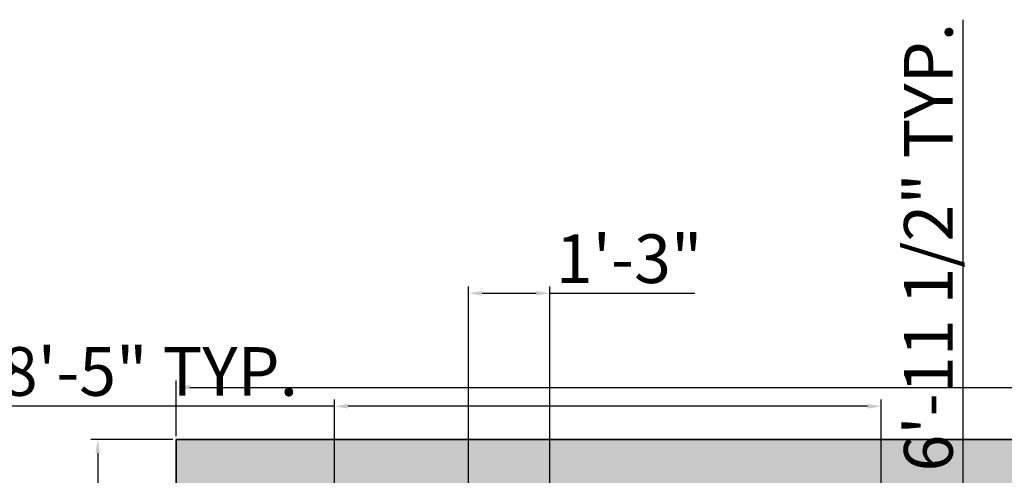
# Model space of a CAD drawing. Units: inches. Extents: x 3592 to 4861, y 1650 to 2243.
# Tile 24 of 30: x 4009 to 4191, y 2159 to 2243. Entities that reach past the tile are written whole.
import ezdxf

# ---------------------------------------------------------------- set-up
doc = ezdxf.new("R2010")
doc.units = ezdxf.units.IN
doc.layers.add('A-ANNO-DIMS', color=2, linetype='Continuous', lineweight=13)
doc.layers.add('A-WALL', color=7, linetype='Continuous', lineweight=35)
doc.layers.add('A-WALL-PATT', color=252, linetype='Continuous', lineweight=13, true_color=0x939598)
doc.styles.get("Standard").update_dxf_attribs({"font": 'arial.ttf'})
doc.dimstyles.new('ISO-25', dxfattribs={"dimtxt": 9, "dimasz": 2.5, "dimexe": 1.25, "dimexo": 0.625, "dimtad": 1, "dimlunit": 3, "dimtxsty": 'Standard', "dimcen": 2.5, "dimadec": 0, "dimazin": 0, "dimtfac": 1, "dimtmove": 0, "dimatfit": 3, "dimfxl": 1, "dimarcsym": 0})

# ---------------------------------------------------------------- blocks, each defined once
blk = doc.blocks.new('*D7')
at = {"layer": 'A-ANNO-DIMS', "color": 0, "lineweight": -2, "transparency": 16777216}
for p, q in [((4038.37, 2165.84), (4038.37, 2176.13)), ((4398.37, 2165.84), (4398.37, 2176.13)), ((4040.87, 2174.88), (4395.87, 2174.88))]:
    blk.add_line(p, q, dxfattribs=at)
at = {"layer": 'A-ANNO-DIMS', "color": 0, "transparency": 16777216}
for points in [[(4040.87, 2175.3), (4040.87, 2174.46), (4038.37, 2174.88)], [(4395.87, 2175.3), (4395.87, 2174.46), (4398.37, 2174.88)]]:
    blk.add_solid(points, dxfattribs=at)
at = {"layer": 'Defpoints', "color": 0, "transparency": 16777216}
for p in [(4398.37, 2174.88), (4038.37, 2165.22), (4398.37, 2165.22)]:
    blk.add_point(p, dxfattribs=at)
at = {"layer": 'A-ANNO-DIMS', "color": 0, "transparency": 16777216, "insert": (4218.37, 2180.1), "char_height": 9, "attachment_point": 5}
blk.add_mtext("30'", dxfattribs=at)
blk = doc.blocks.new('*D6')
at = {"layer": 'A-ANNO-DIMS', "color": 0, "lineweight": -2, "transparency": 16777216}
for p, q in [((4037.74, 2165.22), (4022.59, 2165.22)), ((4023.84, 2162.72), (4023.84, 1687.72)), ((4037.74, 1685.22), (4022.59, 1685.22))]:
    blk.add_line(p, q, dxfattribs=at)
at = {"layer": 'A-ANNO-DIMS', "color": 0, "transparency": 16777216}
for points in [[(4023.43, 2162.72), (4024.26, 2162.72), (4023.84, 2165.22)], [(4023.43, 1687.72), (4024.26, 1687.72), (4023.84, 1685.22)]]:
    blk.add_solid(points, dxfattribs=at)
at = {"layer": 'Defpoints', "color": 0, "transparency": 16777216}
for p in [(4038.37, 2165.22), (4023.84, 1685.22), (4038.37, 1685.22)]:
    blk.add_point(p, dxfattribs=at)
at = {"layer": 'A-ANNO-DIMS', "color": 0, "transparency": 16777216, "insert": (4018.62, 1925.22), "char_height": 9, "attachment_point": 5, "rotation": 90}
blk.add_mtext("40'", dxfattribs=at)
blk = doc.blocks.new('*D154')
at = {"layer": 'A-ANNO-DIMS', "color": 0, "lineweight": -2, "transparency": 16777216}
for p, q in [((4067.61, 2156.84), (4067.61, 2172.62)), ((4168.62, 2156.84), (4168.62, 2172.62)), ((4067.61, 2171.37), (3930.45, 2171.37)), ((4166.12, 2171.37), (4070.11, 2171.37))]:
    blk.add_line(p, q, dxfattribs=at)
at = {"layer": 'A-ANNO-DIMS', "color": 0, "transparency": 16777216}
for points in [[(4070.11, 2171.79), (4070.11, 2170.95), (4067.61, 2171.37)], [(4166.12, 2171.79), (4166.12, 2170.95), (4168.62, 2171.37)]]:
    blk.add_solid(points, dxfattribs=at)
at = {"layer": 'Defpoints', "color": 0, "transparency": 16777216}
for p in [(4067.61, 2171.37), (4067.61, 2156.22), (4168.62, 2156.22)]:
    blk.add_point(p, dxfattribs=at)
at = {"layer": 'A-ANNO-DIMS', "color": 0, "transparency": 16777216, "insert": (3997.78, 2176.65), "char_height": 9, "attachment_point": 5}
blk.add_mtext('BED GROUP 8\'-5" TYP.', dxfattribs=at)
blk = doc.blocks.new('*D155')
at = {"layer": 'A-ANNO-DIMS', "color": 0, "lineweight": -2, "transparency": 16777216}
for p, q in [((4183.77, 2156.22), (4183.77, 2242.84)), ((4169.25, 2156.22), (4185.02, 2156.22)), ((4183.77, 2075.11), (4183.77, 2153.72)), ((4169.25, 2072.61), (4185.02, 2072.61))]:
    blk.add_line(p, q, dxfattribs=at)
at = {"layer": 'A-ANNO-DIMS', "color": 0, "transparency": 16777216}
for points in [[(4183.36, 2153.72), (4184.19, 2153.72), (4183.77, 2156.22)], [(4183.36, 2075.11), (4184.19, 2075.11), (4183.77, 2072.61)]]:
    blk.add_solid(points, dxfattribs=at)
at = {"layer": 'Defpoints', "color": 0, "transparency": 16777216}
for p in [(4168.62, 2156.22), (4183.77, 2156.22), (4168.62, 2072.61)]:
    blk.add_point(p, dxfattribs=at)
at = {"layer": 'A-ANNO-DIMS', "color": 0, "transparency": 16777216, "insert": (4178.5, 2200.78), "char_height": 9, "attachment_point": 5, "rotation": 90}
blk.add_mtext('6\'-11 1/2" TYP.', dxfattribs=at)
blk = doc.blocks.new('*D179')
at = {"layer": 'A-ANNO-DIMS', "color": 0, "lineweight": -2, "transparency": 16777216}
for p, q in [((4092.37, 2010.81), (4092.37, 2193.52)), ((4107.37, 2020.84), (4107.37, 2193.52)), ((4094.87, 2192.27), (4104.87, 2192.27)), ((4107.37, 2192.27), (4134.2, 2192.27))]:
    blk.add_line(p, q, dxfattribs=at)
at = {"layer": 'A-ANNO-DIMS', "color": 0, "transparency": 16777216}
for points in [[(4094.87, 2192.69), (4094.87, 2191.85), (4092.37, 2192.27)], [(4104.87, 2192.69), (4104.87, 2191.85), (4107.37, 2192.27)]]:
    blk.add_solid(points, dxfattribs=at)
at = {"layer": 'Defpoints', "color": 0, "transparency": 16777216}
for p in [(4107.37, 2192.27), (4107.37, 2020.22), (4092.37, 2010.18)]:
    blk.add_point(p, dxfattribs=at)
at = {"layer": 'A-ANNO-DIMS', "color": 0, "transparency": 16777216, "insert": (4122.03, 2197.49), "char_height": 9, "attachment_point": 5}
blk.add_mtext('1\'-3"', dxfattribs=at)

msp = doc.modelspace()

# ---------------------------------------------------------------- hatches: boundary and pattern name
at = {"layer": 'A-WALL-PATT'}
h = msp.add_hatch(color=256, dxfattribs=at)
h.dxf.hatch_style = 1
h.paths.add_polyline_path([(4398.37, 2165.219), (4038.37, 2165.219), (4038.37, 1993.219), (4047.37, 1993.219), (4047.37, 2156.219), (4191.37, 2156.219), (4191.37, 2150.219), (4195.37, 2150.219), (4195.37, 2156.219), (4256.37, 2156.219), (4256.37, 2150.219), (4265.37, 2150.219), (4265.37, 2156.219), (4389.37, 2156.219), (4389.37, 2114.219), (4398.37, 2114.219)])
h.paths.add_polyline_path([(4265.37, 2102.219), (4256.37, 2102.219), (4256.37, 2096.219), (4195.37, 2096.219), (4195.37, 2102.219), (4191.37, 2102.219), (4191.37, 2020.219), (4195.37, 2020.219), (4195.37, 2087.219), (4256.37, 2087.219), (4256.37, 2020.219), (4306.37, 2020.219), (4306.37, 2024.219), (4265.37, 2024.219)], flags=17)
h.paths.add_polyline_path([(4398.37, 2066.219), (4389.37, 2066.219), (4389.37, 2024.219), (4348.37, 2024.219), (4348.37, 2020.219), (4389.37, 2020.219), (4389.37, 1989.719), (4398.37, 1989.719)])
h.paths.add_polyline_path([(4398.37, 1941.719), (4389.37, 1941.719), (4389.37, 1911.219), (4301.37, 1911.219), (4301.37, 1907.219), (4389.37, 1907.219), (4389.37, 1865.219), (4398.37, 1865.219)])
h.paths.add_polyline_path([(4398.37, 1817.219), (4389.37, 1817.219), (4389.37, 1775.219), (4265.37, 1775.219), (4265.37, 1911.219), (4256.37, 1911.219), (4256.37, 1817.219), (4220.87, 1817.219), (4220.87, 1808.219), (4256.37, 1808.219), (4256.37, 1766.219), (4389.37, 1766.219), (4389.37, 1694.219), (4256.37, 1694.219), (4256.37, 1685.219), (4398.37, 1685.219)])
h.paths.add_polyline_path([(4178.87, 1817.219), (4077.37, 1817.219), (4077.37, 1808.219), (4178.87, 1808.219)])
h.paths.add_polyline_path([(4111.37, 2020.219), (4155.37, 2020.219), (4155.37, 2024.219), (4077.37, 2024.219), (4077.37, 2020.219), (4107.37, 2020.219), (4107.37, 1942.219), (4047.37, 1942.219), (4047.37, 1969.219), (4038.37, 1969.219), (4038.37, 1911.219), (4047.37, 1911.219), (4047.37, 1938.219), (4107.37, 1938.219), (4107.37, 1860.219), (4077.37, 1860.219), (4077.37, 1856.219), (4111.37, 1856.219)])
h.paths.add_polyline_path([(4047.37, 1887.219), (4038.37, 1887.219), (4038.37, 1685.219), (4152.37, 1685.219), (4152.37, 1715.219), (4143.37, 1715.219), (4143.37, 1694.219), (4047.37, 1694.219)])
h.paths.add_polyline_path([(4152.37, 1772.219), (4143.37, 1772.219), (4143.37, 1751.219), (4152.37, 1751.219)], flags=17)

# ---------------------------------------------------------------- linework, layer by layer
at = {"layer": 'A-WALL'}
for p, q in [((4038.37, 2165.219), (4398.37, 2165.219)), ((4038.37, 1685.219), (4038.37, 2165.219))]:
    msp.add_line(p, q, dxfattribs=at)

# ---------------------------------------------------------------- dimensions: what is measured, and where the dimension line sits
at = {"layer": 'A-ANNO-DIMS'}
for base, p1, p2, angle, text, picture, middle in [((4183.774, 2156.219), (4168.621, 2072.607), (4168.621, 2156.219), 90, '<> TYP.', '*D155', (4178.495, 2200.78)), ((4067.606, 2171.371), (4168.621, 2156.219), (4067.606, 2156.219), 180, 'BED GROUP <> TYP.', '*D154', (3997.779, 2176.653))]:
    dim = msp.add_linear_dim(base=base, p1=p1, p2=p2, angle=angle, text=text, dimstyle='ISO-25', override={"dimdec": 1, "dimlfac": 1, "dimrnd": 0, "dimzin": 1, "dimdsep": 46, "dimlunit": 4, "dimfrac": 2}, dxfattribs=at)
    dim.commit()
    dim.dimension.update_dxf_attribs({"geometry": picture, "text_midpoint": middle})
for base, p1, p2, override, picture, middle in [((4107.37, 2192.269), (4092.37, 2010.184), (4107.37, 2020.219), {"dimdec": 1, "dimlfac": 1, "dimrnd": 0, "dimzin": 1, "dimdsep": 46, "dimlunit": 4, "dimfrac": 2}, '*D179', (4122.033, 2197.492)), ((4398.37, 2174.88), (4038.37, 2165.219), (4398.37, 2165.219), {"dimclrd": 0, "dimclre": 0, "dimclrt": 0}, '*D7', (4218.37, 2180.103))]:
    dim = msp.add_linear_dim(base=base, p1=p1, p2=p2, dimstyle='ISO-25', override=override, dxfattribs=at)
    dim.commit()
    dim.dimension.update_dxf_attribs({"geometry": picture, "text_midpoint": middle})
dim = msp.add_linear_dim(base=(4023.842, 1685.219), p1=(4038.37, 2165.219), p2=(4038.37, 1685.219), angle=90, dimstyle='ISO-25', override={"dimclrd": 0, "dimclre": 0, "dimclrt": 0}, dxfattribs=at)
dim.commit()
dim.dimension.update_dxf_attribs({"geometry": '*D6', "text_midpoint": (4018.622, 1925.219)})

doc.saveas('drawing.dxf')
